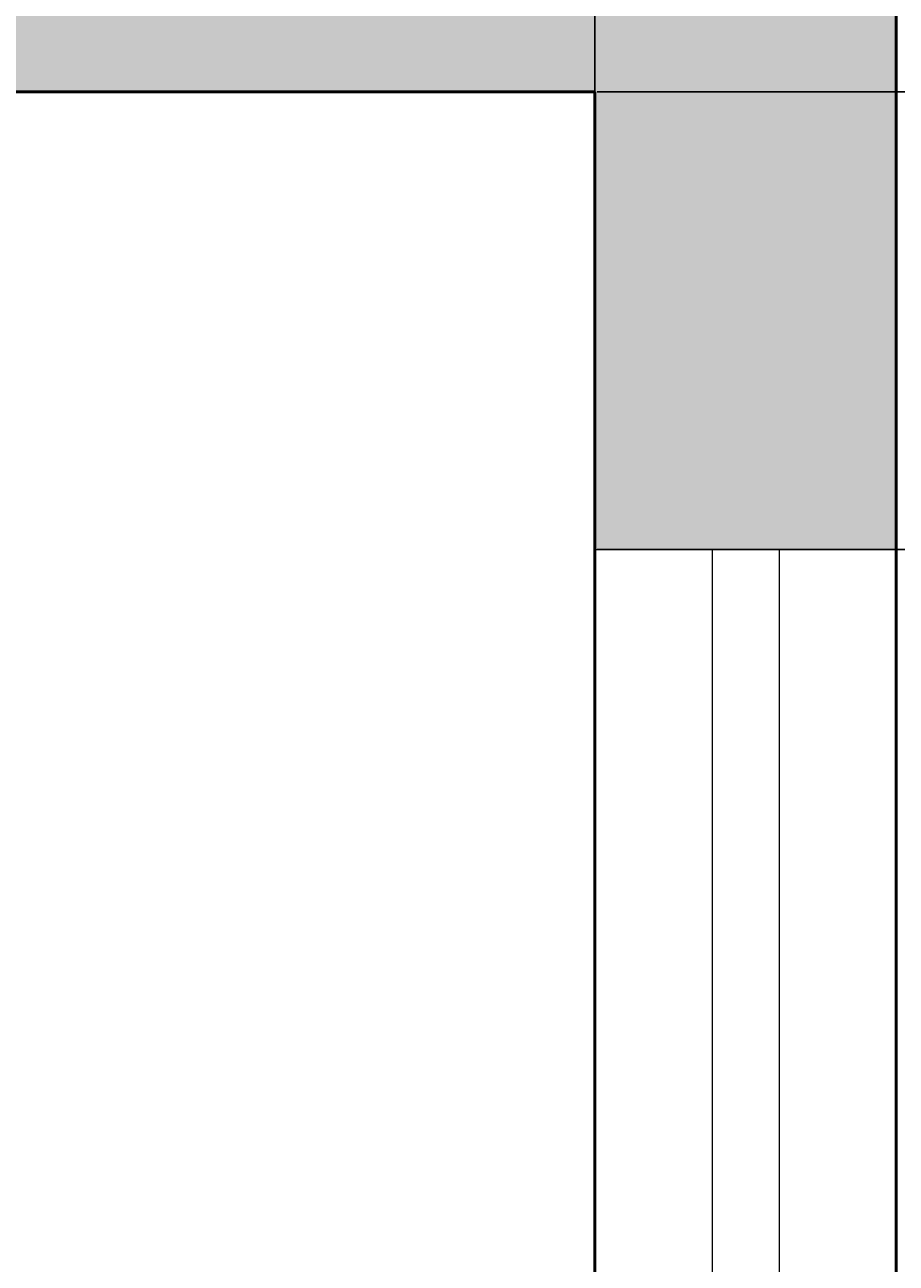
# Model space of a CAD drawing. Units: inches. Extents: x 2231 to 2461, y 2045 to 2455.
# Tile 67 of 95: x 2416 to 2442, y 2296 to 2333. Entities that reach past the tile are written whole.
import ezdxf

# ---------------------------------------------------------------- set-up
doc = ezdxf.new("R2010")
doc.units = ezdxf.units.IN
for name, color, linetype, lineweight in [('A-ANNO-DIMS', 2, 'Continuous', 18), ('A-GLAZ', 4, 'Continuous', 18), ('A-WALL', 7, 'Continuous', 50)]:
    doc.layers.add(name, color=color, linetype=linetype, lineweight=lineweight)
doc.layers.add('A-WALL-PATT', color=18, linetype='Continuous', lineweight=13, true_color=0x000000)
doc.styles.get("Standard").update_dxf_attribs({"font": 'arial.ttf'})
doc.dimstyles.get("Standard").update_dxf_attribs({"dimtxt": 0.18, "dimasz": 0.18, "dimexe": 0.18, "dimexo": 0.0625, "dimgap": 0.09, "dimtad": 0, "dimtih": 1, "dimtoh": 1, "dimdec": 4, "dimzin": 0, "dimdsep": 46, "dimtxsty": 'Standard', "dimcen": 0.09, "dimadec": 0, "dimazin": 0, "dimtfac": 1, "dimtdec": 4, "dimtofl": 0, "dimtmove": 0, "dimatfit": 3, "dimfxl": 1, "dimtolj": 1, "dimtzin": 0, "dimarcsym": 0})

# ---------------------------------------------------------------- blocks, each defined once
blk = doc.blocks.new('WIN-48IN')
for p, q in [((0, 0), (0, 9)), ((0, 5.5), (48, 5.5)), ((0, 3.5), (48, 3.5))]:
    blk.add_line(p, q)
blk = doc.blocks.new('*D42')
at = {"layer": 'A-ANNO-DIMS', "color": 0, "lineweight": -2, "transparency": 16777216}
for p, q in [((2396.794, 2286.895), (2396.794, 2454.645)), ((2432.794, 2286.895), (2432.794, 2454.645)), ((2396.974, 2454.465), (2414.575, 2454.465)), ((2432.614, 2454.465), (2415.012, 2454.465))]:
    blk.add_line(p, q, dxfattribs=at)
at = {"layer": 'A-ANNO-DIMS', "color": 0, "transparency": 16777216}
for points in [[(2396.974, 2454.495), (2396.974, 2454.435), (2396.794, 2454.465)], [(2432.614, 2454.495), (2432.614, 2454.435), (2432.794, 2454.465)]]:
    blk.add_solid(points, dxfattribs=at)
at = {"layer": 'Defpoints', "color": 0, "transparency": 16777216}
for p in [(2432.794, 2454.465), (2396.794, 2286.833), (2432.794, 2286.833)]:
    blk.add_point(p, dxfattribs=at)
at = {"layer": 'A-ANNO-DIMS', "color": 0, "transparency": 16777216, "insert": (2414.794, 2454.465), "char_height": 0.18, "attachment_point": 5}
blk.add_mtext('\\A1;36', dxfattribs=at)
blk = doc.blocks.new('*D58')
at = {"layer": 'A-ANNO-DIMS', "color": 0, "lineweight": -2, "transparency": 16777216}
for p, q in [((2432.856, 2330.833), (2460.606, 2330.833)), ((2460.426, 2330.653), (2460.426, 2324.175)), ((2460.426, 2317.334), (2460.426, 2323.811)), ((2432.856, 2317.154), (2460.606, 2317.154))]:
    blk.add_line(p, q, dxfattribs=at)
at = {"layer": 'A-ANNO-DIMS', "color": 0, "transparency": 16777216}
for points in [[(2460.396, 2330.653), (2460.456, 2330.653), (2460.426, 2330.833)], [(2460.396, 2317.334), (2460.456, 2317.334), (2460.426, 2317.154)]]:
    blk.add_solid(points, dxfattribs=at)
at = {"layer": 'Defpoints', "color": 0, "transparency": 16777216}
for p in [(2432.794, 2330.833), (2432.794, 2317.154), (2460.426, 2317.154)]:
    blk.add_point(p, dxfattribs=at)
at = {"layer": 'A-ANNO-DIMS', "color": 0, "transparency": 16777216, "insert": (2460.426, 2323.993), "char_height": 0.18, "attachment_point": 5}
blk.add_mtext('\\A1;13.68', dxfattribs=at)
blk = doc.blocks.new('*D59')
at = {"layer": 'A-ANNO-DIMS', "color": 0, "lineweight": -2, "transparency": 16777216}
for p, q in [((2408.794, 2182.895), (2408.794, 2454.645)), ((2432.794, 2182.895), (2432.794, 2454.645)), ((2408.974, 2454.465), (2420.573, 2454.465)), ((2432.614, 2454.465), (2421.014, 2454.465))]:
    blk.add_line(p, q, dxfattribs=at)
at = {"layer": 'A-ANNO-DIMS', "color": 0, "transparency": 16777216}
for points in [[(2408.974, 2454.495), (2408.974, 2454.435), (2408.794, 2454.465)], [(2432.614, 2454.495), (2432.614, 2454.435), (2432.794, 2454.465)]]:
    blk.add_solid(points, dxfattribs=at)
at = {"layer": 'Defpoints', "color": 0, "transparency": 16777216}
for p in [(2432.794, 2454.465), (2408.794, 2182.833), (2432.794, 2182.833)]:
    blk.add_point(p, dxfattribs=at)
at = {"layer": 'A-ANNO-DIMS', "color": 0, "transparency": 16777216, "insert": (2420.794, 2454.465), "char_height": 0.18, "attachment_point": 5}
blk.add_mtext('\\A1;24', dxfattribs=at)

msp = doc.modelspace()

# ---------------------------------------------------------------- hatches: boundary and pattern name
at = {"layer": 'A-WALL-PATT'}
h = msp.add_hatch(color=256, dxfattribs=at)
h.dxf.hatch_style = 1
h.paths.add_polyline_path([(2441.7935, 2269.1535), (2432.7935, 2269.1535), (2432.7935, 2186.8328), (2396.7935, 2186.8328), (2396.7935, 2286.8328), (2394.7935, 2286.8328), (2394.7935, 2186.8328), (2334.7935, 2186.8328), (2334.7935, 2182.8328), (2432.7935, 2182.8328), (2432.7935, 2072.8328), (2416.6639, 2072.8328), (2416.6639, 2063.8328), (2441.7935, 2063.8328)])
h.paths.add_polyline_path([(2368.6639, 2072.8328), (2367.04, 2072.8328), (2330.7942, 2072.8328), (2330.7397, 2063.8328), (2368.6639, 2063.8328)])
h.paths.add_polyline_path([(2300.7392, 2068.3328), (2300.7392, 2072.8328), (2298.7935, 2072.8328), (2294.7935, 2072.8328), (2258.7935, 2072.8328), (2258.7935, 2120.8328), (2294.7935, 2120.8328), (2298.7935, 2120.8328), (2298.7935, 2128.8328), (2294.7935, 2128.8328), (2294.7935, 2124.8328), (2258.7935, 2124.8328), (2258.7935, 2182.8328), (2294.7935, 2182.8328), (2294.7935, 2174.8328), (2298.7935, 2174.8328), (2298.7935, 2182.8328), (2304.7935, 2182.8328), (2304.7935, 2186.8328), (2258.7935, 2186.8328), (2258.7935, 2221.999), (2249.7935, 2221.999), (2249.7935, 2063.8328), (2300.7392, 2063.8328)])
h.paths.add_polyline_path([(2391.9338, 2435.8328), (2333.82, 2435.8328), (2333.82, 2426.8328), (2368.7935, 2426.8328), (2368.7935, 2374.9508), (2368.7935, 2370.8328), (2372.3935, 2370.8328), (2372.7935, 2370.8328), (2372.7935, 2426.8328), (2391.9338, 2426.8328)])
h.paths.add_polyline_path([(2441.7935, 2435.8328), (2415.9338, 2435.8328), (2415.9338, 2426.8328), (2432.7935, 2426.8328), (2432.7935, 2334.8328), (2372.7935, 2334.8328), (2372.7935, 2346.8328), (2368.7935, 2346.8328), (2368.7935, 2306.8328), (2360.7935, 2306.8328), (2360.7935, 2302.8328), (2368.7935, 2302.8328), (2372.7935, 2302.8328), (2372.7935, 2330.8328), (2432.7935, 2330.8328), (2432.7935, 2317.1535), (2441.7935, 2317.1535)])
h.paths.add_polyline_path([(2285.82, 2435.8328), (2249.7935, 2435.8328), (2249.7935, 2269.999), (2258.7935, 2269.999), (2258.7935, 2302.8328), (2318.8168, 2302.8328), (2330.7935, 2302.8328), (2330.7935, 2306.8328), (2258.7935, 2306.8328), (2258.7935, 2426.8328), (2285.82, 2426.8328)])

# ---------------------------------------------------------------- linework, layer by layer
at = {"layer": 'A-WALL'}
for p, q in [((2372.7935, 2330.8328), (2432.7935, 2330.8328)), ((2432.7935, 2330.8328), (2432.7935, 2186.8328)), ((2432.7935, 2330.8328), (2432.7935, 2306.8328))]:
    msp.add_line(p, q, dxfattribs=at)
msp.add_lwpolyline([(2300.7392, 2063.8328), (2249.7935, 2063.8328), (2249.7935, 2435.8328), (2441.7935, 2435.8328), (2441.7935, 2063.8328), (2330.7397, 2063.8328)], dxfattribs=at)

# ---------------------------------------------------------------- block references
at = {"layer": 'A-GLAZ', "rotation": 270.0000000000023}
msp.add_blockref('WIN-48IN', (2432.7937, 2317.1535), dxfattribs=at)

# ---------------------------------------------------------------- dimensions: what is measured, and where the dimension line sits
at = {"layer": 'A-ANNO-DIMS'}
for p1, p2, picture, middle in [((2396.7935, 2286.8328), (2432.7935, 2286.8328), '*D42', (2414.7935, 2454.4653)), ((2408.7935, 2182.8328), (2432.7935, 2182.8328), '*D59', (2420.7935, 2454.4653))]:
    dim = msp.add_linear_dim(base=(2432.7935, 2454.4653), p1=p1, p2=p2, dimstyle='Standard', override={"dimdec": 0, "dimlfac": 1, "dimrnd": 0, "dimzin": 0, "dimdsep": 46, "dimlunit": 2}, dxfattribs=at)
    dim.commit()
    dim.dimension.update_dxf_attribs({"geometry": picture, "text_midpoint": middle})
dim = msp.add_linear_dim(base=(2460.426, 2317.1535), p1=(2432.7935, 2330.8328), p2=(2432.7935, 2317.1535), angle=90, dimstyle='Standard', override={"dimdec": 2, "dimlfac": 1, "dimrnd": 0, "dimzin": 0, "dimdsep": 46, "dimlunit": 2}, dxfattribs=at)
dim.commit()
dim.dimension.update_dxf_attribs({"geometry": '*D58', "text_midpoint": (2460.426, 2323.9932)})

doc.saveas('drawing.dxf')
